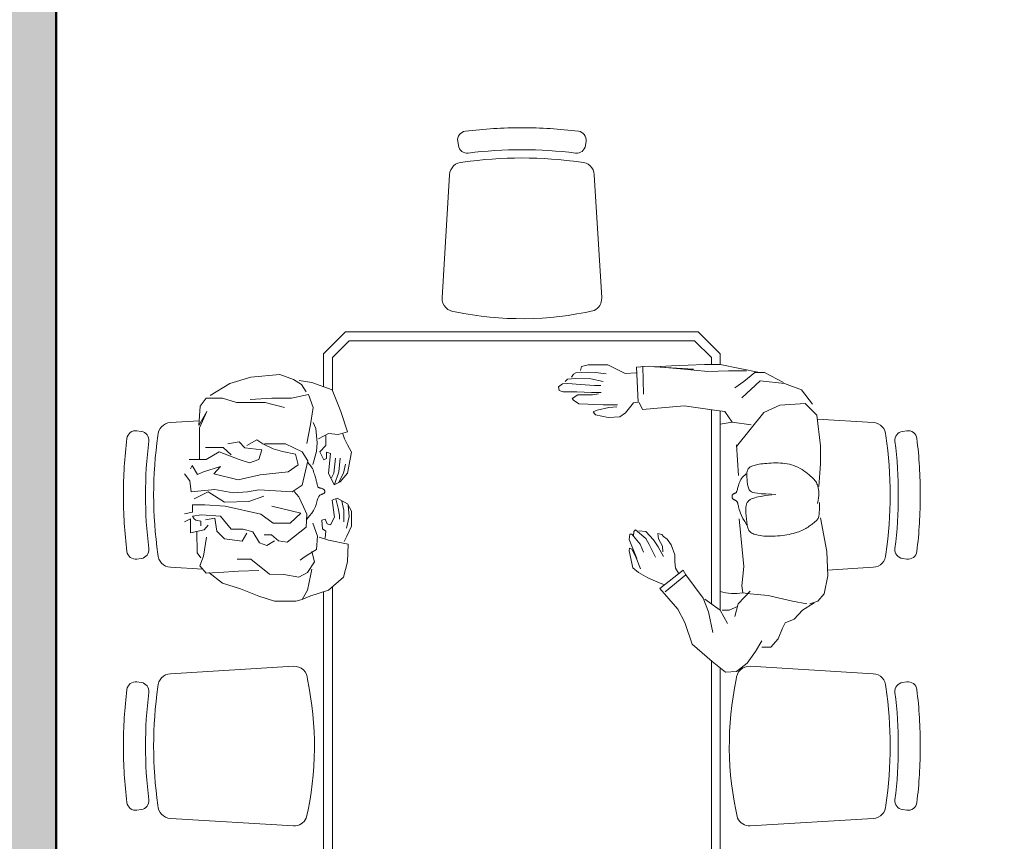
# Model space of a CAD drawing. Units: inches. Extents: x 1734 to 4011, y 1071 to 1891.
# Tile 7 of 27: x 1954 to 2022, y 1699 to 1756. Entities that reach past the tile are written whole.
import ezdxf

# ---------------------------------------------------------------- set-up
doc = ezdxf.new("R2010")
doc.units = ezdxf.units.IN
for name, color, linetype, lineweight in [('A-FURN', 8, 'Continuous', 18), ('A-WALL', 7, 'Continuous', 50), ('A-WALL-PATT', 8, 'Continuous', 13)]:
    doc.layers.add(name, color=color, linetype=linetype, lineweight=lineweight)

# ---------------------------------------------------------------- blocks, each defined once
blk = doc.blocks.new('A$C421907B3')
for p, q in [((0.3928, 1.2157), (0.4173, 1.234)), ((0.4173, 1.234), (0.4418, 1.2361)), ((0.4418, 1.2361), (0.4726, 1.2115)), ((0.3742, 1.1891), (0.3928, 1.2157)), ((0.4726, 1.2115), (0.5176, 1.1724)), ((0.36, 1.1646), (0.3742, 1.1891)), ((0.3229, 1.1605), (0.3394, 1.1788)), ((0.3394, 1.1788), (0.36, 1.1787)), ((0.5176, 1.1724), (0.5341, 1.1234)), ((0.3126, 1.1359), (0.3229, 1.1605)), ((0.4808, 1.0989), (0.4706, 1.1459)), ((0.2861, 1.1152), (0.3066, 1.1235)), ((0.3066, 1.1235), (0.3126, 1.1359)), ((0.4378, 1.1255), (0.454, 1.0947)), ((0.5341, 1.1234), (0.5503, 1.0926)), ((0.2676, 1.0948), (0.2861, 1.1152)), ((0.4132, 1.0806), (0.4212, 1.1093)), ((0.493, 1.0681), (0.4808, 1.0989)), ((0.2328, 1.0745), (0.2183, 1.0579)), ((0.2511, 1.0807), (0.2328, 1.0745)), ((0.241, 1.0786), (0.2676, 1.0948)), ((0.2573, 1.0807), (0.2901, 1.0744)), ((0.2901, 1.0744), (0.3454, 1.062)), ((0.3864, 1.0516), (0.4132, 1.0806)), ((0.4335, 1.0947), (0.4152, 1.0865)), ((0.45, 1.0947), (0.4335, 1.0947)), ((0.454, 1.0947), (0.489, 1.0702)), ((0.5503, 1.0926), (0.5914, 1.0456)), ((1.4171, 1.0745), (1.4031, 1.0709)), ((1.4656, 1.0745), (1.4171, 1.0745)), ((1.5014, 1.0634), (1.4656, 1.0745)), ((0.2183, 1.0579), (0.2102, 1.0171)), ((0.3454, 1.062), (0.3864, 1.0578)), ((0.3864, 1.0578), (0.4029, 1.0557)), ((0.4029, 1.0557), (0.4049, 1.0395)), ((0.5322, 1.015), (0.493, 1.0681)), ((0.5791, 1.0535), (0.532, 1.0149)), ((1.3433, 1.0498), (1.3858, 1.0635)), ((1.3858, 1.0635), (1.4011, 1.0699)), ((1.4031, 1.0709), (1.3905, 1.0498)), ((1.5426, 1.0469), (1.5014, 1.0634)), ((0.4049, 1.0395), (0.4006, 0.9963)), ((0.538, 1.0045), (0.5914, 1.0456)), ((0.5958, 1.0315), (0.5832, 1.0366)), ((0.618, 1.0218), (0.5958, 1.0315)), ((1.3094, 1.0205), (1.3433, 1.0498)), ((1.3905, 1.0498), (1.3831, 1.0131)), ((1.5838, 1.034), (1.5426, 1.0469)), ((1.615, 1.0092), (1.5838, 1.034)), ((0.2102, 1.0171), (0.2122, 0.9615)), ((0.532, 1.0149), (0.538, 1.0045)), ((0.5491, 1.0108), (0.5557, 0.9996)), ((0.6395, 1.0092), (0.618, 1.0218)), ((0.6521, 0.9988), (0.6395, 1.0092)), ((1.3001, 0.9856), (1.3094, 1.0205)), ((1.3751, 0.9856), (1.3904, 1.0094)), ((1.3831, 1.0131), (1.3811, 1.0021)), ((1.3904, 1.0094), (1.4104, 1.0204)), ((1.4104, 1.0204), (1.4443, 1.0139)), ((1.4443, 1.0139), (1.4768, 1.013)), ((1.4768, 1.013), (1.5193, 0.979)), ((1.5014, 1.0047), (1.5472, 1.0065)), ((1.5472, 1.0065), (1.5918, 1.0092)), ((1.5918, 1.0092), (1.621, 1.011)), ((1.621, 1.011), (1.6349, 0.9945)), ((0.4006, 0.9963), (0.4108, 0.8878)), ((0.5557, 0.9996), (0.5572, 0.9855)), ((0.5572, 0.9855), (0.5572, 0.9693)), ((0.635, 1.001), (0.6461, 0.9722)), ((0.6609, 0.9603), (0.6521, 0.9988)), ((1.2987, 0.9453), (1.3001, 0.9856)), ((1.3811, 0.9617), (1.3751, 0.9856)), ((1.6349, 0.9945), (1.627, 0.9725)), ((0.2122, 0.9615), (0.2264, 0.8858)), ((0.5572, 0.9693), (0.5653, 0.947)), ((0.5832, 0.9729), (0.595, 0.9515)), ((0.5854, 0.9499), (0.5846, 0.9626)), ((0.6009, 0.9744), (0.615, 0.9462)), ((0.6283, 0.9633), (0.6357, 0.9455)), ((0.6609, 0.9344), (0.6432, 0.9774)), ((0.6461, 0.9722), (0.655, 0.9566)), ((1.3705, 0.9571), (1.3877, 0.9681)), ((1.3877, 0.9681), (1.3984, 0.9745)), ((1.3984, 0.9745), (1.4077, 0.9819)), ((1.5193, 0.979), (1.5505, 0.979)), ((1.627, 0.9725), (1.6196, 0.9294)), ((1.6409, 0.9652), (1.6329, 0.9762)), ((1.6421, 0.9163), (1.6409, 0.9652)), ((0.5653, 0.947), (0.5742, 0.9337)), ((0.5942, 0.933), (0.5854, 0.9499)), ((0.595, 0.9515), (0.6053, 0.9352)), ((0.615, 0.9462), (0.6232, 0.9322)), ((0.6357, 0.9455), (0.655, 0.9225)), ((0.655, 0.9566), (0.6602, 0.9544)), ((0.6602, 0.9544), (0.6609, 0.9603)), ((1.3432, 0.9361), (1.2987, 0.9453)), ((1.3013, 0.9269), (1.3073, 0.9388)), ((1.3678, 0.9269), (1.3705, 0.9571)), ((1.3937, 0.9067), (1.4369, 0.9406)), ((1.4369, 0.9406), (1.4568, 0.9378)), ((1.4655, 0.9378), (1.4827, 0.9479)), ((1.4827, 0.9479), (1.4994, 0.9423)), ((1.4994, 0.9423), (1.5146, 0.9176)), ((1.5286, 0.9203), (1.5392, 0.9386)), ((1.5392, 0.9386), (1.5791, 0.9331)), ((0.2723, 0.9155), (0.2759, 0.9169)), ((0.2759, 0.9169), (0.2797, 0.9183)), ((0.2797, 0.9183), (0.2839, 0.9196)), ((0.2839, 0.9196), (0.2883, 0.9208)), ((0.2883, 0.9208), (0.2929, 0.922)), ((0.2929, 0.922), (0.2977, 0.923)), ((0.2977, 0.923), (0.3027, 0.924)), ((0.3027, 0.924), (0.3078, 0.9248)), ((0.3078, 0.9248), (0.3131, 0.9255)), ((0.3131, 0.9255), (0.3184, 0.9261)), ((0.3184, 0.9261), (0.3238, 0.9266)), ((0.3238, 0.9266), (0.3293, 0.927)), ((0.3293, 0.927), (0.3347, 0.9272)), ((0.3347, 0.9272), (0.34, 0.9272)), ((0.34, 0.9272), (0.3452, 0.9272)), ((0.3452, 0.9272), (0.3502, 0.927)), ((0.3502, 0.927), (0.355, 0.9267)), ((0.355, 0.9267), (0.3595, 0.9262)), ((0.3595, 0.9262), (0.3638, 0.9257)), ((0.3638, 0.9257), (0.3677, 0.925)), ((0.3677, 0.925), (0.3713, 0.9242)), ((0.3713, 0.9242), (0.3746, 0.9233)), ((0.3746, 0.9233), (0.3776, 0.9223)), ((0.3776, 0.9223), (0.3803, 0.9212)), ((0.3803, 0.9212), (0.3826, 0.92)), ((0.3826, 0.92), (0.3847, 0.9187)), ((0.3847, 0.9187), (0.3864, 0.9173)), ((0.3864, 0.9173), (0.3878, 0.9158)), ((0.5742, 0.9337), (0.5832, 0.9278)), ((0.5832, 0.9278), (0.5869, 0.9233)), ((0.5869, 0.9233), (0.5957, 0.9211)), ((0.5957, 0.9211), (0.5942, 0.933)), ((0.6053, 0.9352), (0.6232, 0.9166)), ((0.6232, 0.9322), (0.6461, 0.9129)), ((0.6232, 0.9166), (0.6387, 0.9151)), ((0.6461, 0.9129), (0.6498, 0.9166)), ((0.6498, 0.9166), (0.6506, 0.9263)), ((0.655, 0.9225), (0.6594, 0.9225)), ((0.6594, 0.9225), (0.6609, 0.9344)), ((1.2907, 0.904), (1.3013, 0.9269)), ((1.3645, 0.9296), (1.3432, 0.9361)), ((1.3505, 0.9315), (1.3492, 0.9159)), ((1.3784, 0.8975), (1.3678, 0.9269)), ((1.4568, 0.9378), (1.4721, 0.924)), ((1.4721, 0.924), (1.4887, 0.924)), ((1.5146, 0.9176), (1.5365, 0.9111)), ((1.5791, 0.9331), (1.5963, 0.9157)), ((1.6256, 0.9129), (1.6561, 0.9193)), ((1.6561, 0.9193), (1.6561, 0.8881)), ((0.237, 0.8927), (0.2385, 0.8941)), ((0.2385, 0.8941), (0.2401, 0.8956)), ((0.2401, 0.8956), (0.2419, 0.897)), ((0.2419, 0.897), (0.2437, 0.8985)), ((0.2437, 0.8985), (0.2457, 0.9)), ((0.2457, 0.9), (0.2478, 0.9016)), ((0.2478, 0.9016), (0.25, 0.9031)), ((0.25, 0.9031), (0.2524, 0.9047)), ((0.2524, 0.9047), (0.2548, 0.9063)), ((0.2548, 0.9063), (0.2573, 0.9078)), ((0.2573, 0.9078), (0.26, 0.9094)), ((0.26, 0.9094), (0.2628, 0.911)), ((0.2628, 0.911), (0.2657, 0.9125)), ((0.2657, 0.9125), (0.2689, 0.914)), ((0.2689, 0.914), (0.2723, 0.9155)), ((0.3878, 0.9158), (0.389, 0.9142)), ((0.389, 0.9142), (0.39, 0.9123)), ((0.39, 0.9123), (0.3908, 0.9104)), ((0.3908, 0.9104), (0.3915, 0.9081)), ((0.3915, 0.9081), (0.3921, 0.9057)), ((0.3921, 0.9057), (0.3926, 0.903)), ((0.3926, 0.903), (0.3931, 0.8999)), ((0.3931, 0.8999), (0.3935, 0.8967)), ((0.3935, 0.8967), (0.394, 0.8933)), ((0.3936, 0.9023), (0.3986, 0.894)), ((0.3986, 0.894), (0.4026, 0.8867)), ((1.2906, 0.87), (1.2907, 0.904)), ((1.2965, 0.8821), (1.3022, 0.9091)), ((1.3079, 0.8681), (1.3079, 0.8945)), ((1.3385, 0.9012), (1.3292, 0.8838)), ((1.3458, 0.8994), (1.3385, 0.9012)), ((1.3505, 0.8883), (1.3458, 0.8994)), ((1.3492, 0.9159), (1.3565, 0.9104)), ((1.3565, 0.9104), (1.3584, 0.8911)), ((1.3923, 0.8773), (1.3937, 0.9067)), ((1.4056, 0.8745), (1.4302, 0.8974)), ((1.4302, 0.8974), (1.4687, 0.8974)), ((1.4687, 0.8974), (1.4966, 0.8772)), ((1.5365, 0.9111), (1.5638, 0.9111)), ((1.5638, 0.9111), (1.5883, 0.8817)), ((1.5963, 0.9157), (1.601, 0.8863)), ((1.6163, 0.9019), (1.6256, 0.9129)), ((1.6329, 0.8927), (1.6329, 0.9037)), ((1.6561, 0.8881), (1.6701, 0.8945)), ((0.2291, 0.8687), (0.2292, 0.8722)), ((0.2292, 0.8722), (0.2294, 0.8753)), ((0.2294, 0.8753), (0.2297, 0.8781)), ((0.2297, 0.8781), (0.2301, 0.8806)), ((0.2301, 0.8806), (0.2306, 0.8828)), ((0.2306, 0.8828), (0.2313, 0.8848)), ((0.2313, 0.8848), (0.2322, 0.8866)), ((0.2322, 0.8866), (0.2332, 0.8883)), ((0.2332, 0.8883), (0.2343, 0.8898)), ((0.2343, 0.8898), (0.2356, 0.8913)), ((0.2356, 0.8913), (0.237, 0.8927)), ((0.394, 0.8933), (0.3944, 0.8898)), ((0.3944, 0.8898), (0.3947, 0.8863)), ((0.3947, 0.8863), (0.3951, 0.8829)), ((0.3951, 0.8829), (0.3954, 0.8796)), ((0.3954, 0.8796), (0.3957, 0.8765)), ((0.3957, 0.8765), (0.3959, 0.8736)), ((0.3959, 0.8736), (0.3961, 0.871)), ((0.4026, 0.8867), (0.4057, 0.8804)), ((0.4057, 0.8804), (0.4081, 0.8751)), ((0.4081, 0.8751), (0.4098, 0.8705)), ((1.2985, 0.8577), (1.2965, 0.8821)), ((1.3183, 0.8795), (1.3183, 0.8888)), ((1.3209, 0.8634), (1.3183, 0.8795)), ((1.3292, 0.8838), (1.3351, 0.8452)), ((1.3584, 0.8911), (1.3505, 0.8883)), ((1.3774, 0.869), (1.3812, 0.8747)), ((1.3812, 0.8747), (1.3861, 0.8811)), ((1.3861, 0.8811), (1.3923, 0.8883)), ((1.3996, 0.8608), (1.3923, 0.8773)), ((1.472, 0.8589), (1.4056, 0.8745)), ((1.4966, 0.8772), (1.5777, 0.8588)), ((1.5883, 0.8817), (1.6315, 0.8789)), ((1.601, 0.8863), (1.6222, 0.8899)), ((1.6315, 0.8789), (1.6515, 0.8817)), ((1.6442, 0.8908), (1.6329, 0.8927)), ((1.6481, 0.8881), (1.6442, 0.8908)), ((1.6515, 0.8817), (1.6481, 0.8881)), ((1.6514, 0.8725), (1.6701, 0.8761)), ((1.6514, 0.856), (1.6514, 0.8725)), ((0.2291, 0.8649), (0.2291, 0.8687)), ((0.2291, 0.8607), (0.2291, 0.8649)), ((0.2291, 0.856), (0.2291, 0.8607)), ((0.2291, 0.8509), (0.2291, 0.856)), ((0.2316, 0.8463), (0.2331, 0.8527)), ((0.3918, 0.8495), (0.3909, 0.8482)), ((0.3927, 0.8508), (0.3918, 0.8495)), ((0.3934, 0.8523), (0.3927, 0.8508)), ((0.3941, 0.8538), (0.3934, 0.8523)), ((0.3947, 0.8553), (0.3941, 0.8538)), ((0.3952, 0.857), (0.3947, 0.8553)), ((0.3956, 0.8587), (0.3952, 0.857)), ((0.3959, 0.8604), (0.3956, 0.8587)), ((0.3961, 0.8623), (0.3959, 0.8604)), ((0.3961, 0.871), (0.3962, 0.8685)), ((0.3962, 0.8642), (0.3961, 0.8623)), ((0.3962, 0.8685), (0.3962, 0.8663)), ((0.3962, 0.8663), (0.3962, 0.8642)), ((0.4098, 0.8705), (0.411, 0.8667)), ((0.411, 0.8667), (0.4118, 0.8634)), ((0.4118, 0.8634), (0.4124, 0.8607)), ((0.4124, 0.8607), (0.4129, 0.8583)), ((0.4129, 0.8583), (0.4134, 0.8564)), ((0.4134, 0.8564), (0.4138, 0.8547)), ((0.4138, 0.8547), (0.4141, 0.8533)), ((0.4141, 0.8533), (0.4145, 0.8522)), ((0.4145, 0.8522), (0.4148, 0.8512)), ((0.4148, 0.8512), (0.4152, 0.8504)), ((0.4152, 0.8504), (0.4156, 0.8497)), ((0.4156, 0.8497), (0.416, 0.849)), ((1.2999, 0.8535), (1.2906, 0.87)), ((1.3232, 0.8407), (1.2999, 0.8535)), ((1.3126, 0.8473), (1.3079, 0.8681)), ((1.3261, 0.8427), (1.3209, 0.8634)), ((1.3694, 0.849), (1.3702, 0.852)), ((1.3702, 0.852), (1.3712, 0.8555)), ((1.3712, 0.8555), (1.3726, 0.8595)), ((1.3726, 0.8595), (1.3746, 0.864)), ((1.3746, 0.864), (1.3774, 0.869)), ((1.4102, 0.8378), (1.3996, 0.8608)), ((1.5239, 0.8487), (1.579, 0.8496)), ((1.5777, 0.8588), (1.6235, 0.856)), ((1.579, 0.8496), (1.6162, 0.8266)), ((1.6235, 0.856), (1.6514, 0.856)), ((0.2301, 0.8299), (0.2302, 0.8349)), ((0.2304, 0.8252), (0.2301, 0.8299)), ((0.2302, 0.8349), (0.2307, 0.8404)), ((0.2307, 0.8404), (0.2316, 0.8463)), ((0.3369, 0.8333), (0.328, 0.8326)), ((0.3448, 0.8341), (0.3369, 0.8333)), ((0.3375, 0.8319), (0.3508, 0.8313)), ((0.3518, 0.835), (0.3448, 0.8341)), ((0.3508, 0.8313), (0.3614, 0.8306)), ((0.3579, 0.8359), (0.3518, 0.835)), ((0.3632, 0.8369), (0.3579, 0.8359)), ((0.3614, 0.8306), (0.3695, 0.8298)), ((0.3678, 0.8379), (0.3632, 0.8369)), ((0.3718, 0.8389), (0.3678, 0.8379)), ((0.3695, 0.8298), (0.3757, 0.8289)), ((0.3752, 0.8398), (0.3718, 0.8389)), ((0.3782, 0.8407), (0.3752, 0.8398)), ((0.3757, 0.8289), (0.3801, 0.8278)), ((0.3807, 0.8416), (0.3782, 0.8407)), ((0.3801, 0.8278), (0.3832, 0.8265)), ((0.3829, 0.8425), (0.3807, 0.8416)), ((0.3847, 0.8433), (0.3829, 0.8425)), ((0.3863, 0.8442), (0.3847, 0.8433)), ((0.3876, 0.8451), (0.3863, 0.8442)), ((0.3888, 0.846), (0.3876, 0.8451)), ((0.3899, 0.8471), (0.3888, 0.846)), ((0.3909, 0.8482), (0.3899, 0.8471)), ((0.416, 0.849), (0.4165, 0.8484)), ((0.4165, 0.8484), (0.417, 0.8478)), ((0.4173, 0.827), (0.4168, 0.826)), ((0.417, 0.8478), (0.4176, 0.8473)), ((0.4178, 0.8277), (0.4173, 0.827)), ((0.4176, 0.8473), (0.4182, 0.8468)), ((0.4183, 0.8283), (0.4178, 0.8277)), ((0.4182, 0.8468), (0.4188, 0.8463)), ((0.4188, 0.8288), (0.4183, 0.8283)), ((0.4188, 0.8463), (0.4195, 0.8459)), ((0.4194, 0.8291), (0.4188, 0.8288)), ((0.42, 0.8294), (0.4194, 0.8291)), ((0.4195, 0.8459), (0.4202, 0.8455)), ((0.4207, 0.8297), (0.42, 0.8294)), ((0.4202, 0.8455), (0.4209, 0.8451)), ((0.4215, 0.83), (0.4207, 0.8297)), ((0.4209, 0.8451), (0.4217, 0.8448)), ((0.4223, 0.8303), (0.4215, 0.83)), ((0.4217, 0.8448), (0.4225, 0.8444)), ((0.4231, 0.8307), (0.4223, 0.8303)), ((0.4225, 0.8444), (0.4233, 0.8439)), ((0.424, 0.8311), (0.4231, 0.8307)), ((0.4233, 0.8439), (0.424, 0.8435)), ((0.424, 0.8435), (0.4247, 0.8429)), ((0.4248, 0.8316), (0.424, 0.8311)), ((0.4247, 0.8429), (0.4253, 0.8423)), ((0.4255, 0.8322), (0.4248, 0.8316)), ((0.4253, 0.8423), (0.4259, 0.8415)), ((0.4261, 0.8329), (0.4255, 0.8322)), ((0.4259, 0.8415), (0.4264, 0.8407)), ((0.4267, 0.8337), (0.4261, 0.8329)), ((0.4264, 0.8407), (0.4268, 0.8397)), ((0.427, 0.8346), (0.4267, 0.8337)), ((0.4268, 0.8397), (0.4271, 0.8387)), ((0.4272, 0.8356), (0.427, 0.8346)), ((0.4271, 0.8387), (0.4273, 0.8377)), ((0.4273, 0.8366), (0.4272, 0.8356)), ((0.4273, 0.8377), (0.4273, 0.8366)), ((1.3351, 0.8452), (1.3232, 0.8407)), ((1.3512, 0.826), (1.3514, 0.8269)), ((1.3514, 0.8269), (1.3518, 0.8277)), ((1.3518, 0.8277), (1.3524, 0.8285)), ((1.3524, 0.8285), (1.353, 0.8292)), ((1.353, 0.8292), (1.3538, 0.8299)), ((1.3538, 0.8299), (1.3547, 0.8305)), ((1.3547, 0.8305), (1.3557, 0.8311)), ((1.3557, 0.8311), (1.3568, 0.8316)), ((1.3568, 0.8316), (1.3579, 0.832)), ((1.3579, 0.832), (1.3591, 0.8325)), ((1.3591, 0.8325), (1.3602, 0.833)), ((1.3602, 0.833), (1.3613, 0.8335)), ((1.3613, 0.8335), (1.3624, 0.8342)), ((1.3624, 0.8342), (1.3634, 0.835)), ((1.3634, 0.835), (1.3643, 0.8359)), ((1.3643, 0.8359), (1.3651, 0.837)), ((1.3651, 0.837), (1.3659, 0.8384)), ((1.3659, 0.8384), (1.3666, 0.8399)), ((1.3666, 0.8399), (1.3673, 0.8417)), ((1.3673, 0.8417), (1.368, 0.8438)), ((1.368, 0.8438), (1.3687, 0.8462)), ((1.3687, 0.8462), (1.3694, 0.849)), ((1.4029, 0.8112), (1.4255, 0.8268)), ((1.4208, 0.8259), (1.4102, 0.8378)), ((1.4255, 0.8268), (1.5012, 0.8222)), ((1.49, 0.8359), (1.5239, 0.8487)), ((1.5272, 0.8267), (1.5591, 0.8285)), ((1.5591, 0.8285), (1.6009, 0.8212)), ((1.6162, 0.8266), (1.6481, 0.8422)), ((0.2306, 0.814), (0.2263, 0.7628)), ((0.2309, 0.821), (0.2304, 0.8252)), ((0.2316, 0.8172), (0.2309, 0.821)), ((0.2325, 0.8138), (0.2316, 0.8172)), ((0.2335, 0.8107), (0.2325, 0.8138)), ((0.2346, 0.8079), (0.2335, 0.8107)), ((0.2359, 0.8053), (0.2346, 0.8079)), ((0.2374, 0.8029), (0.2359, 0.8053)), ((0.3832, 0.8265), (0.3854, 0.8251)), ((0.3854, 0.8251), (0.3869, 0.8235)), ((0.3869, 0.8235), (0.3882, 0.8218)), ((0.3882, 0.8218), (0.3892, 0.8198)), ((0.3892, 0.8198), (0.3901, 0.8176)), ((0.3901, 0.8176), (0.3908, 0.8153)), ((0.3908, 0.8153), (0.3914, 0.8128)), ((0.3914, 0.8128), (0.3919, 0.8101)), ((0.3919, 0.8101), (0.3923, 0.8073)), ((0.3923, 0.8073), (0.3926, 0.8043)), ((0.4108, 0.8066), (0.4098, 0.804)), ((0.4117, 0.8093), (0.4108, 0.8066)), ((0.4126, 0.8119), (0.4117, 0.8093)), ((0.4133, 0.8145), (0.4126, 0.8119)), ((0.414, 0.8169), (0.4133, 0.8145)), ((0.4147, 0.8192), (0.414, 0.8169)), ((0.4152, 0.8213), (0.4147, 0.8192)), ((0.4158, 0.8231), (0.4152, 0.8213)), ((0.4163, 0.8247), (0.4158, 0.8231)), ((0.4168, 0.826), (0.4163, 0.8247)), ((1.3089, 0.784), (1.3203, 0.8058)), ((1.3165, 0.804), (1.3305, 0.8104)), ((1.3193, 0.7809), (1.3297, 0.8099)), ((1.3305, 0.8104), (1.3431, 0.7838)), ((1.3512, 0.8251), (1.3512, 0.826)), ((1.3514, 0.8243), (1.3512, 0.8251)), ((1.3518, 0.8234), (1.3514, 0.8243)), ((1.3524, 0.8226), (1.3518, 0.8234)), ((1.3531, 0.8218), (1.3524, 0.8226)), ((1.354, 0.8211), (1.3531, 0.8218)), ((1.355, 0.8204), (1.354, 0.8211)), ((1.3561, 0.8198), (1.355, 0.8204)), ((1.3572, 0.8192), (1.3561, 0.8198)), ((1.3584, 0.8188), (1.3572, 0.8192)), ((1.3595, 0.8184), (1.3584, 0.8188)), ((1.3607, 0.8181), (1.3595, 0.8184)), ((1.3618, 0.8179), (1.3607, 0.8181)), ((1.3629, 0.8176), (1.3618, 0.8179)), ((1.3639, 0.8173), (1.3629, 0.8176)), ((1.3648, 0.8169), (1.3639, 0.8173)), ((1.3656, 0.8165), (1.3648, 0.8169)), ((1.3664, 0.8159), (1.3656, 0.8165)), ((1.367, 0.8151), (1.3664, 0.8159)), ((1.3675, 0.8141), (1.367, 0.8151)), ((1.3679, 0.813), (1.3675, 0.8141)), ((1.3683, 0.8118), (1.3679, 0.813)), ((1.3686, 0.8104), (1.3683, 0.8118)), ((1.369, 0.8088), (1.3686, 0.8104)), ((1.3694, 0.8071), (1.369, 0.8088)), ((1.3698, 0.8053), (1.3694, 0.8071)), ((1.3703, 0.8033), (1.3698, 0.8053)), ((1.3902, 0.7562), (1.4029, 0.8112)), ((1.5012, 0.8222), (1.5272, 0.8267)), ((1.6009, 0.8212), (1.6547, 0.8266)), ((1.6547, 0.8266), (1.6574, 0.8018)), ((0.2391, 0.8006), (0.2374, 0.8029)), ((0.241, 0.7983), (0.2391, 0.8006)), ((0.2433, 0.7958), (0.241, 0.7983)), ((0.246, 0.7933), (0.2433, 0.7958)), ((0.249, 0.7905), (0.246, 0.7933)), ((0.2523, 0.7876), (0.249, 0.7905)), ((0.256, 0.7846), (0.2523, 0.7876)), ((0.2599, 0.7816), (0.256, 0.7846)), ((0.3926, 0.8043), (0.393, 0.8012)), ((0.393, 0.8012), (0.3933, 0.7979)), ((0.3934, 0.7825), (0.393, 0.7799)), ((0.3933, 0.7979), (0.3936, 0.7947)), ((0.3937, 0.7853), (0.3934, 0.7825)), ((0.3936, 0.7947), (0.3937, 0.7915)), ((0.3937, 0.7915), (0.3938, 0.7883)), ((0.3938, 0.7883), (0.3937, 0.7853)), ((0.3986, 0.7884), (0.3953, 0.7859)), ((0.4014, 0.7909), (0.3986, 0.7884)), ((0.4037, 0.7935), (0.4014, 0.7909)), ((0.4057, 0.796), (0.4037, 0.7935)), ((0.4073, 0.7987), (0.4057, 0.796)), ((0.4087, 0.8013), (0.4073, 0.7987)), ((0.4098, 0.804), (0.4087, 0.8013)), ((0.413, 0.7893), (0.417, 0.7199)), ((1.2905, 0.7361), (1.2999, 0.7838)), ((1.2999, 0.7838), (1.3165, 0.804)), ((1.3047, 0.7638), (1.3089, 0.784)), ((1.3275, 0.7498), (1.3307, 0.784)), ((1.3307, 0.784), (1.3359, 0.7949)), ((1.3431, 0.7838), (1.3384, 0.7397)), ((1.3708, 0.8013), (1.3703, 0.8033)), ((1.3714, 0.799), (1.3708, 0.8013)), ((1.3721, 0.7967), (1.3714, 0.799)), ((1.3728, 0.7942), (1.3721, 0.7967)), ((1.3736, 0.7916), (1.3728, 0.7942)), ((1.3743, 0.7889), (1.3736, 0.7916)), ((1.3751, 0.786), (1.3743, 0.7889)), ((1.376, 0.783), (1.3751, 0.786)), ((1.3769, 0.7799), (1.376, 0.783)), ((1.4348, 0.7809), (1.4979, 0.7882)), ((1.4979, 0.7882), (1.5484, 0.7992)), ((1.5484, 0.7992), (1.6035, 0.7854)), ((1.6035, 0.7854), (1.5882, 0.7689)), ((1.6268, 0.7808), (1.6407, 0.7872)), ((1.6407, 0.7872), (1.6527, 0.767)), ((1.6574, 0.8018), (1.67, 0.7853)), ((0.2263, 0.7628), (0.2263, 0.7217)), ((0.264, 0.7786), (0.2599, 0.7816)), ((0.2684, 0.7758), (0.264, 0.7786)), ((0.2729, 0.7731), (0.2684, 0.7758)), ((0.2776, 0.7707), (0.2729, 0.7731)), ((0.2823, 0.7686), (0.2776, 0.7707)), ((0.2871, 0.7668), (0.2823, 0.7686)), ((0.292, 0.7652), (0.2871, 0.7668)), ((0.297, 0.764), (0.292, 0.7652)), ((0.302, 0.7629), (0.297, 0.764)), ((0.3071, 0.7621), (0.302, 0.7629)), ((0.3123, 0.7616), (0.3071, 0.7621)), ((0.3176, 0.7612), (0.3123, 0.7616)), ((0.3229, 0.7609), (0.3176, 0.7612)), ((0.3282, 0.7609), (0.3229, 0.7609)), ((0.3335, 0.7609), (0.3282, 0.7609)), ((0.3387, 0.7611), (0.3335, 0.7609)), ((0.3438, 0.7614), (0.3387, 0.7611)), ((0.3486, 0.7618), (0.3438, 0.7614)), ((0.3533, 0.7622), (0.3486, 0.7618)), ((0.3576, 0.7627), (0.3533, 0.7622)), ((0.3617, 0.7632), (0.3576, 0.7627)), ((0.3654, 0.7637), (0.3617, 0.7632)), ((0.3688, 0.7643), (0.3654, 0.7637)), ((0.3719, 0.7649), (0.3688, 0.7643)), ((0.3748, 0.7656), (0.3719, 0.7649)), ((0.3774, 0.7663), (0.3748, 0.7656)), ((0.3799, 0.7671), (0.3774, 0.7663)), ((0.3821, 0.768), (0.3799, 0.7671)), ((0.3841, 0.7689), (0.3821, 0.768)), ((0.386, 0.7699), (0.3841, 0.7689)), ((0.3876, 0.7711), (0.386, 0.7699)), ((0.3891, 0.7724), (0.3876, 0.7711)), ((0.3904, 0.7739), (0.3891, 0.7724)), ((0.3914, 0.7756), (0.3904, 0.7739)), ((0.3923, 0.7776), (0.3914, 0.7756)), ((0.393, 0.7799), (0.3923, 0.7776)), ((1.3166, 0.7498), (1.3193, 0.7809)), ((1.3703, 0.7351), (1.3783, 0.7645)), ((1.378, 0.7767), (1.3769, 0.7799)), ((1.3795, 0.7735), (1.378, 0.7767)), ((1.3813, 0.7701), (1.3795, 0.7735)), ((1.3837, 0.7667), (1.3813, 0.7701)), ((1.3866, 0.7633), (1.3837, 0.7667)), ((1.3902, 0.7599), (1.3866, 0.7633)), ((1.4122, 0.7654), (1.4348, 0.7809)), ((1.4181, 0.7406), (1.4122, 0.7654)), ((1.5012, 0.7534), (1.5224, 0.7607)), ((1.5224, 0.7607), (1.5457, 0.7533)), ((1.5882, 0.7689), (1.6268, 0.7808)), ((1.6527, 0.767), (1.656, 0.7743)), ((1.3384, 0.7397), (1.3477, 0.7361)), ((1.3477, 0.7507), (1.3537, 0.7535)), ((1.3477, 0.7361), (1.3477, 0.7507)), ((1.3537, 0.7535), (1.363, 0.736)), ((1.4028, 0.736), (1.3902, 0.7562)), ((1.4473, 0.7351), (1.4181, 0.7406)), ((1.4945, 0.7313), (1.5012, 0.7534)), ((1.5457, 0.7533), (1.5915, 0.7358)), ((1.5822, 0.7258), (1.5636, 0.7423)), ((1.5915, 0.7358), (1.6208, 0.7532)), ((1.6208, 0.7532), (1.6593, 0.7532)), ((1.6361, 0.7532), (1.636, 0.6808)), ((0.2263, 0.7217), (0.2345, 0.6523)), ((0.3554, 0.646), (0.417, 0.7237)), ((1.2998, 0.7196), (1.2905, 0.7361)), ((1.3071, 0.7058), (1.2998, 0.7196)), ((1.363, 0.736), (1.349, 0.7214)), ((1.349, 0.7214), (1.349, 0.6984)), ((1.3689, 0.7149), (1.3703, 0.7351)), ((1.3842, 0.6736), (1.3922, 0.7167)), ((1.4407, 0.7176), (1.4028, 0.736)), ((1.4885, 0.7176), (1.4407, 0.7176)), ((1.4686, 0.7286), (1.4473, 0.7351)), ((1.4918, 0.7176), (1.4686, 0.7286)), ((1.5058, 0.7084), (1.4918, 0.7176)), ((1.5331, 0.7267), (1.4945, 0.7313)), ((1.5284, 0.7212), (1.5058, 0.7084)), ((1.5457, 0.7129), (1.5331, 0.7267)), ((1.5716, 0.7175), (1.5457, 0.7129)), ((1.6221, 0.7257), (1.5822, 0.7258)), ((1.2998, 0.6902), (1.3211, 0.6966)), ((1.3104, 0.6948), (1.3071, 0.7058)), ((1.3211, 0.6966), (1.343, 0.6939)), ((1.343, 0.6939), (1.3656, 0.7058)), ((1.3716, 0.6828), (1.3689, 0.7149)), ((0.3842, 0.6746), (0.4272, 0.6684)), ((0.4272, 0.6684), (0.4542, 0.6729)), ((1.315, 0.6443), (1.2998, 0.6902)), ((1.3782, 0.6691), (1.3716, 0.6828)), ((1.3782, 0.6351), (1.3842, 0.6736)), ((1.636, 0.6808), (1.6194, 0.6441)), ((1.6194, 0.6441), (1.6373, 0.6762)), ((1.6373, 0.6762), (1.6346, 0.6321)), ((0.2345, 0.6523), (0.261, 0.6256)), ((0.4272, 0.6684), (0.4435, 0.6438)), ((0.6692, 0.647), (0.6821, 0.6561)), ((0.6821, 0.6561), (0.7085, 0.6576)), ((0.7085, 0.6576), (0.7372, 0.6515)), ((0.7372, 0.6515), (0.7425, 0.6447)), ((0.2448, 0.6277), (0.2693, 0.5949)), ((0.261, 0.6256), (0.3186, 0.6294)), ((0.3186, 0.6294), (0.3554, 0.646)), ((0.4435, 0.6438), (0.462, 0.6418)), ((0.462, 0.6418), (0.5358, 0.6313)), ((0.5358, 0.6313), (0.6302, 0.6396)), ((0.6302, 0.6396), (0.6381, 0.6233)), ((0.6511, 0.6244), (0.6692, 0.647)), ((0.6873, 0.6288), (0.7199, 0.6288)), ((0.707, 0.6349), (0.6889, 0.6334)), ((0.7335, 0.6409), (0.707, 0.6349)), ((0.7199, 0.6288), (0.741, 0.6281)), ((0.7425, 0.6447), (0.7335, 0.6409)), ((0.741, 0.6281), (0.7546, 0.6273)), ((0.7546, 0.6273), (0.775, 0.6265)), ((0.775, 0.6265), (0.787, 0.6183)), ((1.3349, 0.5948), (1.315, 0.6443)), ((1.3888, 0.6057), (1.3782, 0.6351)), ((1.4871, 0.624), (1.4426, 0.6351)), ((1.6346, 0.6321), (1.6207, 0.6138)), ((0.3636, 0.5741), (0.4047, 0.6131)), ((0.6281, 0.6047), (0.6301, 0.5411)), ((0.6405, 0.6229), (0.6511, 0.6244)), ((0.6405, 0.6229), (0.6444, 0.5432)), ((0.744, 0.6062), (0.7304, 0.6039)), ((0.7621, 0.6062), (0.744, 0.6062)), ((0.7772, 0.6062), (0.7621, 0.6062)), ((0.7901, 0.6144), (0.7772, 0.6062)), ((0.787, 0.6183), (0.7901, 0.6144)), ((1.4273, 0.614), (1.3888, 0.6057)), ((1.4718, 0.6139), (1.4273, 0.614)), ((1.521, 0.6166), (1.4718, 0.6139)), ((1.5516, 0.624), (1.4871, 0.624)), ((1.5835, 0.6138), (1.5516, 0.624)), ((1.6114, 0.6074), (1.5668, 0.5808)), ((1.6207, 0.6138), (1.5835, 0.6138)), ((0.2693, 0.5949), (0.3083, 0.5804)), ((0.4004, 0.5761), (0.4209, 0.5906)), ((0.7243, 0.6009), (0.7462, 0.6009)), ((0.7395, 0.585), (0.7251, 0.585)), ((0.7712, 0.5828), (0.7395, 0.585)), ((0.7462, 0.6009), (0.7795, 0.5993)), ((0.7999, 0.5804), (0.7712, 0.5828)), ((0.7795, 0.5993), (0.8105, 0.5993)), ((0.8119, 0.5812), (0.7999, 0.5804)), ((0.8105, 0.5993), (0.8195, 0.5963)), ((0.8211, 0.588), (0.8119, 0.5812)), ((0.8195, 0.5963), (0.8211, 0.588)), ((1.3808, 0.5782), (1.3349, 0.5948)), ((1.404, 0.5828), (1.3934, 0.5993)), ((1.4226, 0.5718), (1.404, 0.5828)), ((0.3083, 0.5804), (0.3636, 0.5741)), ((0.3103, 0.5783), (0.3533, 0.5558)), ((0.3759, 0.5558), (0.4004, 0.5761)), ((0.7198, 0.576), (0.7477, 0.5699)), ((0.7477, 0.5699), (0.7825, 0.5691)), ((0.7817, 0.5563), (0.787, 0.5593)), ((0.7825, 0.5691), (0.8006, 0.5707)), ((0.787, 0.5593), (0.7916, 0.5661)), ((0.8006, 0.5707), (0.8059, 0.576)), ((1.41, 0.5736), (1.3808, 0.5782)), ((1.4532, 0.5598), (1.4226, 0.5718)), ((1.519, 0.5662), (1.4532, 0.5598)), ((1.5668, 0.5808), (1.519, 0.5662)), ((0.3533, 0.5558), (0.3759, 0.5558)), ((0.4543, 0.5377), (0.3646, 0.5558)), ((0.4354, 0.5516), (0.3944, 0.5516)), ((0.4825, 0.5536), (0.4354, 0.5516)), ((0.544, 0.5474), (0.4825, 0.5536)), ((0.6156, 0.5411), (0.544, 0.5474)), ((0.6444, 0.5432), (0.6156, 0.5411)), ((0.645, 0.5564), (0.6699, 0.5579)), ((0.6699, 0.5579), (0.6926, 0.5466)), ((0.6926, 0.5466), (0.7092, 0.5382)), ((0.7092, 0.5382), (0.7538, 0.5382)), ((0.713, 0.5586), (0.7372, 0.5555)), ((0.7372, 0.5555), (0.756, 0.5548)), ((0.7538, 0.5382), (0.7689, 0.5419)), ((0.756, 0.5548), (0.7817, 0.5563)), ((0.7689, 0.5419), (0.7711, 0.551))]:
    blk.add_line(p, q)
at = {"ltscale": 0.1}
for points in [[(0.4542, 1.2262), (0.4542, 2.2936), (0.5042, 2.3436), (0.5562, 2.3436)], [(1.2446, 2.3436), (1.3042, 2.3436), (1.3542, 2.2936), (1.3542, 1.0533)], [(0.4742, 1.2101), (0.4742, 2.2853), (0.5125, 2.3236), (0.5723, 2.3236)], [(1.245, 2.3234), (1.2959, 2.3236), (1.3342, 2.2853), (1.3342, 1.0419)], [(0.4542, 0.6426), (0.4542, 1.0946)], [(0.4742, 0.64), (0.4742, 1.0806)], [(1.3542, 0.5878), (1.3542, 0.5135), (1.3042, 0.4635), (0.5042, 0.4635), (0.4542, 0.5135), (0.4542, 0.5377)], [(1.3342, 0.5966), (1.3342, 0.5218), (1.2959, 0.4835), (0.5125, 0.4835), (0.4742, 0.5218), (0.4742, 0.5375)]]:
    blk.add_lwpolyline(points, dxfattribs=at)
for points in [[(0.0782, 1.5378, -0.399285), (0.1067, 1.5678), (0.3861, 1.5847, -0.305593), (0.4148, 1.5674, -0.109362), (0.4176, 1.2524, -0.429301), (0.3861, 1.2224), (0.1067, 1.2393, -0.399285), (0.0782, 1.2693, -0.071734)], [(1.7302, 1.5378, 0.399285), (1.7017, 1.5678), (1.4223, 1.5847, 0.305593), (1.3936, 1.5674, 0.109362), (1.3908, 1.2524, 0.429301), (1.4223, 1.2224), (1.7017, 1.2393, 0.399285), (1.7302, 1.2693, 0.071734)], [(0.05, 1.4036, 0.030867), (0.0575, 1.2816, -0.408428), (0.0405, 1.2593), (0.0306, 1.2579, -0.419966), (0.0079, 1.2752, -0.030916), (0, 1.4036, -0.030916), (0.0079, 1.5319, -0.419966), (0.0306, 1.5492), (0.0405, 1.5478, -0.408428), (0.0575, 1.5255, 0.030867)], [(1.7584, 1.4036, -0.030867), (1.7509, 1.2816, 0.408428), (1.7679, 1.2593), (1.7778, 1.2579, 0.419966), (1.8005, 1.2752, 0.030916), (1.8084, 1.4036, 0.030916), (1.8005, 1.5319, 0.419966), (1.7778, 1.5492), (1.7679, 1.5478, 0.408428), (1.7509, 1.5255, -0.030867)], [(0.05, 0.8335, -0.030867), (0.0575, 0.9554, 0.408428), (0.0405, 0.9777), (0.0306, 0.9791, 0.419966), (0.0079, 0.9618, 0.030916), (0, 0.8335, 0.030916), (0.0079, 0.7052, 0.419966), (0.0306, 0.6878), (0.0405, 0.6893, 0.408428), (0.0575, 0.7115, -0.030867)], [(1.7584, 0.8335, 0.030867), (1.7509, 0.9554, -0.408428), (1.7679, 0.9777), (1.7778, 0.9791, -0.419966), (1.8005, 0.9618, -0.030916), (1.8084, 0.8335, -0.030916), (1.8005, 0.7052, -0.419966), (1.7778, 0.6878), (1.7679, 0.6893, -0.408428), (1.7509, 0.7115, 0.030867)], [(0.77, 0.0782, -0.399285), (0.74, 0.1067), (0.7231, 0.3861, -0.305593), (0.7404, 0.4148, -0.109362), (1.0554, 0.4176, -0.429301), (1.0853, 0.3861), (1.0684, 0.1067, -0.399285), (1.0384, 0.0782, -0.071734)], [(0.9042, 0.05, 0.030867), (1.0261, 0.0575, -0.408428), (1.0484, 0.0405), (1.0498, 0.0306, -0.419966), (1.0325, 0.0079, -0.030916), (0.9042, 0, -0.030916), (0.7759, 0.0079, -0.419966), (0.7586, 0.0306), (0.76, 0.0405, -0.408428), (0.7823, 0.0575, 0.030867)]]:
    blk.add_lwpolyline(points, format="xyb", close=True, dxfattribs=at)
for points in [[(0.2107, 1.004), (0.1067, 0.9977, 0.399285), (0.0782, 0.9677, 0.071734), (0.0782, 0.6992, 0.399285), (0.1067, 0.6693), (0.2334, 0.6616)], [(1.6285, 1.0021), (1.7017, 0.9977, -0.399285), (1.7302, 0.9677, -0.071734), (1.7302, 0.6992, -0.399285), (1.7017, 0.6693), (1.6367, 0.6653)]]:
    blk.add_lwpolyline(points, format="xyb", dxfattribs=at)
blk.add_lwpolyline([(0.5267, 0.5491), (0.5148, 0.5482), (0.6033, 0.5427), (0.6033, 0.5427), (0.5647, 0.5405), (0.5267, 0.5387), (0.4898, 0.5376), (0.4542, 0.5371)])
blk.add_arc((0.4222, 0.9527), 0.1048, 72.2191, 100.5893)

msp = doc.modelspace()

# ---------------------------------------------------------------- hatches: boundary and pattern name
at = {"layer": 'A-WALL-PATT'}
h = msp.add_hatch(color=256, dxfattribs=at)
h.dxf.hatch_style = 1
h.paths.add_polyline_path([(1857.65, 1835.061), (1857.65, 1793.061), (1862.65, 1793.061), (1862.65, 1835.061), (1951.65, 1835.061), (1951.65, 1763.061), (1897.65, 1763.061), (1897.65, 1758.061), (1951.65, 1758.061), (1951.65, 1617.061), (1956.65, 1617.061), (1956.65, 1758.061), (2009.65, 1758.061), (2009.65, 1763.061), (1956.65, 1763.061), (1956.65, 1835.061), (2044.65, 1835.061), (2044.65, 1763.061), (2039.65, 1763.061), (2039.65, 1758.061), (2054.65, 1758.061), (2054.65, 1763.061), (2049.65, 1763.061), (2049.65, 1835.061), (2109.65, 1835.061), (2109.65, 1763.061), (2084.65, 1763.061), (2084.65, 1758.061), (2109.65, 1758.061), (2109.65, 1530.061), (2095.15, 1530.061), (2095.15, 1525.061), (2109.65, 1525.061), (2109.65, 1471.061), (2089.15, 1471.061), (2089.15, 1466.061), (2109.65, 1466.061), (2109.65, 1250.061), (2015.65, 1250.061), (2015.65, 1241.061), (2109.65, 1241.061), (2109.65, 1133.061), (1952.65, 1133.061), (1952.65, 1197.061), (1953.65, 1197.061), (1953.65, 1202.061), (1946.65, 1202.061), (1946.65, 1133.061), (1934.65, 1133.061), (1934.65, 1124.061), (2118.65, 1124.061), (2118.65, 1844.061), (1758.65, 1844.061), (1758.65, 1758.061), (1773.65, 1758.061), (1773.65, 1763.061), (1767.65, 1763.061), (1767.65, 1835.061)])
h.paths.add_polyline_path([(1803.65, 1649.061), (1812.65, 1649.061), (1812.65, 1758.061), (1867.65, 1758.061), (1867.65, 1763.061), (1797.65, 1763.061), (1797.65, 1758.061), (1803.65, 1758.061)], flags=17)
h.paths.add_polyline_path([(1803.65, 1572.061), (1956.65, 1572.061), (1956.65, 1581.061), (1951.65, 1581.061), (1951.65, 1577.061), (1812.65, 1577.061), (1812.65, 1601.061), (1803.65, 1601.061)], flags=17)
h.paths.add_polyline_path([(2044.65, 1530.061), (2044.65, 1525.061), (2059.15, 1525.061), (2059.15, 1530.061)], flags=17)
h.paths.add_polyline_path([(2009.65, 1466.061), (2035.15, 1466.061), (2035.15, 1471.061), (2014.65, 1471.061), (2014.65, 1530.061), (2009.65, 1530.061)], flags=17)
h.paths.add_polyline_path([(1896.65, 1537.061), (1896.65, 1533.061), (1901.65, 1533.061), (1901.65, 1542.061), (1803.65, 1542.061), (1803.65, 1507.061), (1812.65, 1507.061), (1812.65, 1537.061)], flags=17)
h.paths.add_polyline_path([(1906.65, 1466.061), (1906.65, 1471.061), (1901.65, 1471.061), (1901.65, 1503.061), (1896.65, 1503.061), (1896.65, 1471.061), (1812.65, 1471.061), (1812.65, 1483.061), (1803.65, 1483.061), (1803.65, 1400.061), (1812.65, 1400.061), (1812.65, 1466.061)], flags=17)
h.paths.add_polyline_path([(1951.65, 1334.061), (1909.15, 1334.061), (1909.15, 1325.061), (1956.65, 1325.061), (1956.65, 1466.061), (1961.65, 1466.061), (1961.65, 1471.061), (1942.65, 1471.061), (1942.65, 1466.061), (1951.65, 1466.061)], flags=17)
h.paths.add_polyline_path([(1812.65, 1334.061), (1812.65, 1352.061), (1803.65, 1352.061), (1803.65, 1325.061), (1855.15, 1325.061), (1855.15, 1334.061)], flags=17)
h.paths.add_polyline_path([(1956.65, 1298.061), (1956.65, 1301.061), (1947.65, 1301.061), (1947.65, 1298.061)], flags=17)
h.paths.add_polyline_path([(1967.65, 1241.061), (1967.65, 1250.061), (1947.65, 1250.061), (1947.65, 1241.061)], flags=17)

# ---------------------------------------------------------------- linework, layer by layer
at = {"layer": 'A-WALL'}
msp.add_line((1956.65, 1617.061), (1956.65, 1758.061), dxfattribs=at)

# ---------------------------------------------------------------- block references
at = {"layer": 'A-FURN', "xscale": 30.26057373645948, "yscale": 30.26057373645948, "zscale": 30.26057373645948, "rotation": 180}
msp.add_blockref('A$C421907B3', (2015.998, 1748.475), dxfattribs=at)

doc.saveas('drawing.dxf')
